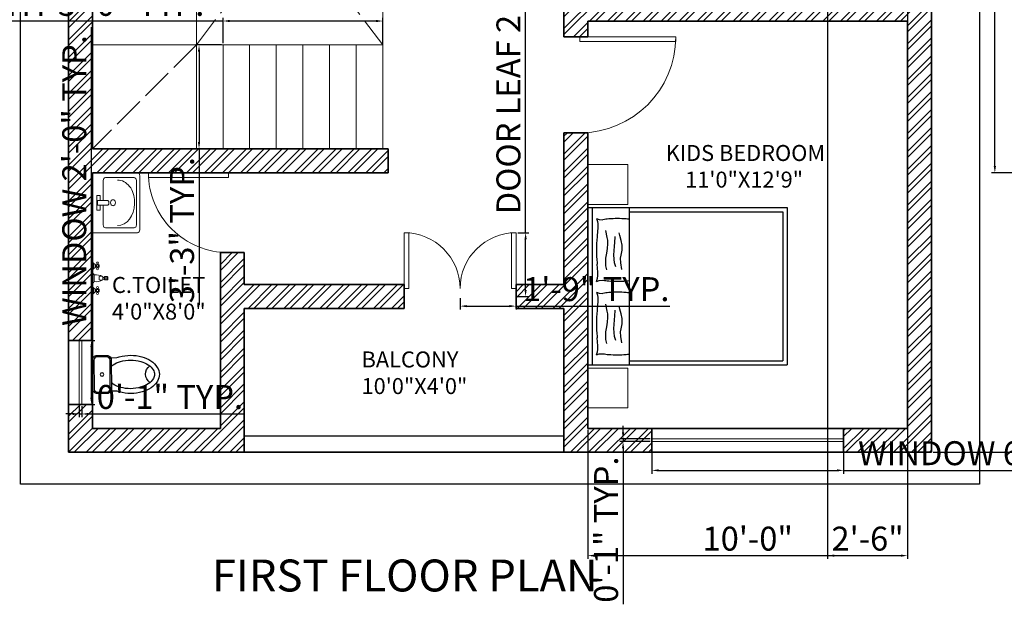
# Model space of a CAD drawing. Units: inches. Extents: x 638 to 1853, y 4393 to 5041.
# Tile 4 of 6: x 1072 to 1441, y 4399 to 4619. Entities that reach past the tile are written whole.
import ezdxf

# ---------------------------------------------------------------- set-up
doc = ezdxf.new("R2010")
doc.units = ezdxf.units.IN
doc.linetypes.add('ACAD_ISO02W100', pattern=[15, 12, -3])
for name, color, linetype, lineweight in [('A-ANNO-DIMS', 2, 'Continuous', 18), ('A-ANNO-TEXT', 7, 'Continuous', 25), ('A-AREA-IDEN', 7, 'Continuous', 18), ('A-DOOR', 4, 'Continuous', 18), ('A-FLOR-FIXT', 9, 'Continuous', 18), ('A-FLOR-STRS', 7, 'Continuous', 18), ('A-FLOR-STRS-HIDN', 7, 'ACAD_ISO02W100', 18), ('A-FURN', 26, 'Continuous', 13), ('A-GLAZ', 5, 'Continuous', 18), ('A-WALL', 7, 'Continuous', 35), ('A-WALL-PATT', 251, 'Continuous', 13), ('A-WALL-PRPT', 7, 'Continuous', 25), ('C-PROP', 7, 'Continuous', 25)]:
    doc.layers.add(name, color=color, linetype=linetype, lineweight=lineweight)
for name, color, linetype in [('SANTEH', 7, 'Continuous'), ('supurgelik', 31, 'Continuous'), ('TASLAR', 32, 'Continuous')]:
    doc.layers.add(name, color=color, linetype=linetype)
doc.styles.get("Standard").update_dxf_attribs({"font": 'arial.ttf'})
doc.dimstyles.new('ISO-25', dxfattribs={"dimtxt": 9, "dimasz": 2.5, "dimexe": 1.25, "dimexo": 0.625, "dimtad": 1, "dimdec": 1, "dimlunit": 3, "dimtxsty": 'Standard', "dimcen": 2.5, "dimadec": 0, "dimazin": 0, "dimtfac": 1, "dimtdec": 1, "dimtmove": 0, "dimatfit": 3, "dimfxl": 1, "dimarcsym": 0})

# ---------------------------------------------------------------- blocks, each defined once
blk = doc.blocks.new('*U2')
for p, q in [((0, 0), (0, -6)), ((-36, 0), (-36, -6))]:
    blk.add_line(p, q)
blk.add_lwpolyline([(0, 0), (0, 36), (-1.75, 36), (-1.75, 0)], close=True)
blk.add_arc((0, 0), 36, 90, 180)
blk = doc.blocks.new('*U3')
for p, q in [((-30, 0), (-30, -6)), ((0, 0), (0, -6))]:
    blk.add_line(p, q)
blk.add_lwpolyline([(0, 0), (0, 30), (-1.75, 30), (-1.75, 0)], close=True)
blk.add_arc((0, 0), 30, 90, 180)
blk = doc.blocks.new('hgjgh')
at = {"layer": 'supurgelik'}
for p, q in [((85993.81, -4751.89), (85843.81, -4751.89)), ((85853.26, -4756.05), (85856.29, -4757)), ((85853.26, -4756.05), (85854.18, -4758.49)), ((85854.18, -4758.49), (85854.49, -4762.19)), ((85856.29, -4757), (85858.52, -4757.5)), ((85858.52, -4757.5), (85862.12, -4757.37)), ((85862.12, -4757.37), (85869.57, -4756.72)), ((85904.4, -4757.37), (85896.95, -4756.72)), ((85908, -4757.5), (85904.4, -4757.37)), ((85910.23, -4757), (85908, -4757.5)), ((85913.26, -4756.05), (85910.23, -4757)), ((85912.34, -4758.49), (85912.03, -4762.19)), ((85913.26, -4756.05), (85912.34, -4758.49)), ((85923.48, -4756.05), (85926.51, -4757)), ((85923.48, -4756.05), (85924.4, -4758.49)), ((85924.4, -4758.49), (85924.71, -4762.19)), ((85926.51, -4757), (85928.74, -4757.5)), ((85928.74, -4757.5), (85932.34, -4757.37)), ((85932.34, -4757.37), (85939.79, -4756.72)), ((85974.62, -4757.37), (85967.17, -4756.72)), ((85978.22, -4757.5), (85974.62, -4757.37)), ((85980.45, -4757), (85978.22, -4757.5)), ((85983.48, -4756.05), (85980.45, -4757)), ((85982.56, -4758.49), (85982.25, -4762.19)), ((85983.48, -4756.05), (85982.56, -4758.49)), ((85864.23, -4765.86), (85867.95, -4764.99)), ((85867.95, -4764.99), (85871.91, -4764.87)), ((85871.91, -4764.87), (85875.39, -4765.12)), ((85875.39, -4765.12), (85878.49, -4765.74)), ((85878.49, -4765.74), (85881.96, -4766.23)), ((85881.96, -4766.23), (85884.81, -4766.61)), ((85884.81, -4766.61), (85888.65, -4766.85)), ((85888.65, -4766.85), (85892.62, -4766.85)), ((85892.62, -4766.85), (85895.1, -4766.36)), ((85895.1, -4766.36), (85901.8, -4764.87)), ((85934.44, -4765.86), (85938.16, -4764.99)), ((85938.16, -4764.99), (85942.13, -4764.87)), ((85942.13, -4764.87), (85945.6, -4765.12)), ((85945.6, -4765.12), (85948.7, -4765.74)), ((85948.7, -4765.74), (85952.18, -4766.23)), ((85952.18, -4766.23), (85955.03, -4766.61)), ((85955.03, -4766.61), (85958.87, -4766.85)), ((85958.87, -4766.85), (85962.84, -4766.85)), ((85962.84, -4766.85), (85965.32, -4766.36)), ((85965.32, -4766.36), (85972.02, -4764.87)), ((85871.29, -4773.05), (85867.33, -4774.04)), ((85870.92, -4779.28), (85875.39, -4779.03)), ((85874.27, -4772.55), (85871.29, -4773.05)), ((85878.86, -4772.3), (85874.27, -4772.55)), ((85875.39, -4779.03), (85878.24, -4779.65)), ((85881.96, -4772.55), (85878.86, -4772.3)), ((85887.04, -4773.05), (85881.96, -4772.55)), ((85890.14, -4773.3), (85887.04, -4773.05)), ((85896.09, -4773.67), (85890.14, -4773.3)), ((85892.37, -4779.65), (85896.96, -4778.41)), ((85896.96, -4778.41), (85899.69, -4777.54)), ((85941.51, -4773.05), (85937.54, -4774.04)), ((85941.14, -4779.28), (85945.6, -4779.03)), ((85944.49, -4772.55), (85941.51, -4773.05)), ((85949.08, -4772.3), (85944.49, -4772.55)), ((85945.6, -4779.03), (85948.46, -4779.65)), ((85952.18, -4772.55), (85949.08, -4772.3)), ((85957.26, -4773.05), (85952.18, -4772.55)), ((85960.36, -4773.3), (85957.26, -4773.05)), ((85966.31, -4773.67), (85960.36, -4773.3)), ((85962.59, -4779.65), (85967.18, -4778.41)), ((85967.18, -4778.41), (85969.91, -4777.54)), ((85993.81, -4787.2), (85843.81, -4787.2)), ((85847.81, -4787.2), (85847.81, -4933.89)), ((85864.72, -4780.15), (85870.92, -4779.28)), ((85878.24, -4779.65), (85882.95, -4780.4)), ((85882.95, -4780.4), (85887.91, -4780.4)), ((85887.91, -4780.4), (85892.37, -4779.65)), ((85934.94, -4780.15), (85941.14, -4779.28)), ((85948.46, -4779.65), (85953.17, -4780.4)), ((85953.17, -4780.4), (85958.13, -4780.4)), ((85958.13, -4780.4), (85962.59, -4779.65)), ((85989.81, -4787.2), (85989.81, -4933.89)), ((85989.81, -4933.89), (85847.81, -4933.89))]:
    blk.add_line(p, q, dxfattribs=at)
for centre, radius, start, end in [((85877.36, -4828.49), 72.19, 95.13619, 96.19323), ((85883.26, -4894.18), 138.14, 90, 95.13619), ((85883.26, -4894.18), 138.14, 84.86381, 90), ((85889.16, -4828.49), 72.19, 83.80677, 84.86381), ((85947.57, -4828.49), 72.19, 95.13619, 96.19323), ((85953.48, -4894.18), 138.14, 90, 95.13619), ((85953.48, -4894.18), 138.14, 84.86381, 90), ((85959.38, -4828.49), 72.19, 83.80677, 84.86381), ((85954.09, -4776.05), 100.71, 175.30047, 180), ((85905.8, -4772.08), 52.26, 169.08956, 175.30047), ((85860.72, -4772.08), 52.26, 4.69953, 10.91044), ((85812.43, -4776.05), 100.71, 0, 4.69953), ((86024.31, -4776.05), 100.71, 175.30047, 180), ((85976.02, -4772.08), 52.26, 169.08956, 175.30047), ((85930.94, -4772.08), 52.26, 4.69953, 10.91044), ((85882.65, -4776.05), 100.71, 0, 4.69953), ((85954.09, -4776.05), 100.71, 180, 184.69953), ((85812.43, -4776.05), 100.71, 355.30047, 0), ((86024.31, -4776.05), 100.71, 180, 184.69953), ((85882.65, -4776.05), 100.71, 355.30047, 0), ((85905.8, -4780.02), 52.26, 184.69953, 187.89725), ((85860.72, -4780.02), 52.26, 352.10275, 355.30047), ((85976.02, -4780.02), 52.26, 184.69953, 187.89725), ((85930.94, -4780.02), 52.26, 352.10275, 355.30047)]:
    blk.add_arc(centre, radius, start, end, dxfattribs=at)
at = {"layer": 'TASLAR'}
for p, q in [((85843.81, -4747.89), (85843.81, -4937.89)), ((85993.81, -4747.89), (85843.81, -4747.89)), ((85993.81, -4747.89), (85993.81, -4937.89)), ((85993.81, -4937.89), (85843.81, -4937.89))]:
    blk.add_line(p, q, dxfattribs=at)
blk = doc.blocks.new('K10-44')
at = {"layer": 'SANTEH'}
for points in [[(-182, 223, 0.020439), (-174, 198), (-174, 135, 0.262987), (-198, 92), (-198, -8, 0.414214), (-148, -58), (152, -58, 0.414214), (202, -8), (202, 92, 0.262987), (178, 135), (178, 198, 0.020439), (186, 223, 0.067459), (202, 342, 0.067459), (186, 461, 0.079812), (143, 554, 0.107118), (74, 621, 0.139889), (2, 642, 0.139889), (-70, 621, 0.107118), (-140, 554, 0.079812), (-182, 461, 0.067459), (-198, 342, 0.067459)], [(-148, 127), (152, 127, -0.414214), (187, 92), (187, -8, -0.414214), (152, -43), (-148, -43, -0.414214), (-183, -8), (-183, 92, -0.414214)]]:
    blk.add_lwpolyline(points, format="xyb", close=True, dxfattribs=at)
for points in [[(90, 142, 0.027307), (102, 158, 0.079812), (137, 236, 0.067459), (152, 342, 0.067459), (137, 448, 0.079812), (102, 526, 0.107118), (47, 579, 0.139889), (2, 592, 0.139889), (-44, 579, 0.107118), (-98, 526, 0.079812), (-134, 448, 0.067459), (-148, 342, 0.067459), (-134, 236, 0.079812), (-98, 158, 0.027307), (-86, 142, 0.139889)], [(-174, 135, -0.136371), (-148, 142), (152, 142, -0.136371), (178, 135)]]:
    blk.add_lwpolyline(points, format="xyb", dxfattribs=at)
blk.add_circle((2, 42), 18.3, dxfattribs=at)
blk.add_arc((2, 602), 105, 213.8994, 326.1006, dxfattribs=at)
blk = doc.blocks.new('Rac7')
at = {"color": 0}
for p, q in [((-39500.6, -24232.1), (-39500.6, -23829.6)), ((-39473.6, -23808.4), (-38988.3, -23808.4)), ((-39456.5, -23859.1), (-39456.5, -24114.9)), ((-39032.4, -23838), (-39429.6, -23838)), ((-39221.1, -23854.9), (-39240.8, -23854.9)), ((-39005.4, -24114.9), (-39005.4, -23859.1)), ((-39005.4, -23859.1), (-39005.4, -23859.1)), ((-38961.3, -23829.6), (-38961.3, -24232.1)), ((-39252.5, -24185.9), (-39252.5, -24093.6)), ((-39209.4, -24185.9), (-39209.4, -24093.6)), ((-39429.6, -24136.1), (-39252.5, -24136.1)), ((-39297, -24164), (-39252.5, -24164)), ((-39297, -24193.5), (-39297, -24164)), ((-39164.9, -24193.5), (-39297, -24193.5)), ((-39252.5, -24185.9), (-39209.4, -24185.9)), ((-39209.4, -24136.1), (-39032.4, -24136.1)), ((-39209.4, -24164), (-39164.9, -24164)), ((-39164.9, -24164), (-39164.9, -24193.5)), ((-38961.3, -24232.1), (-39500.6, -24232.1))]:
    blk.add_line(p, q, dxfattribs=at)
at = {"color": 0, "extrusion": (0, 0, -1)}
for centre, major_axis, start_param, end_param in [((-39473.6, -23829.6), (-27, 0), 0, 1.570796), ((-39429.6, -23859.1), (-27, 0), 0, 1.570796), ((-39240.8, -24007.4), (-194.1, 0), 0, 1.570796), ((-39221.1, -24007.4), (-194.1, 0), 1.570796, 3.141593), ((-39032.4, -23859.1), (-27, 0), 1.570796, 3.141593), ((-38988.3, -23829.6), (-27, 0), 1.570796, 3.141593), ((-39429.6, -24114.9), (-27, 0), -1.570796, 0), ((-39231, -24104), (-25.3, 0), 0.552816, 2.588777), ((-39032.4, -24114.9), (-27, 0), -3.141593, -1.570796)]:
    blk.add_ellipse(centre, major_axis=major_axis, ratio=0.785714, start_param=start_param, end_param=end_param, dxfattribs=at)
blk.add_ellipse((-39231, -24048), major_axis=(-27.9, 0), ratio=0.785714, dxfattribs=at)
blk = doc.blocks.new('Faucet - Bathroom front')
for p, q in [((-0.5, 4.25), (0.5, 4.25)), ((0.5, 3.75), (-0.5, 3.75)), ((-0.5, 3), (0.5, 3)), ((-0.25, 3), (-0.25, 3.5)), ((0.25, 3.5), (0.25, 3)), ((-5, 0), (-2.25, 0)), ((-4.5087, 0.25), (-2.7408, 0.25)), ((-4, 1.625), (-4.25, 1.625)), ((-4, 1.375), (-4.25, 1.375)), ((-3.1442, 0.75), (-4.0979, 0.75)), ((-3.25, 1.625), (-3, 1.625)), ((-3.25, 1.375), (-3, 1.375)), ((-1.5, 0), (1.5, 0)), ((-1, 0.5), (1, 0.5)), ((0.5, 2), (-0.5, 2)), ((2.25, 0), (5, 0)), ((2.7413, 0.25), (4.5092, 0.25)), ((3.25, 1.625), (3, 1.625)), ((3.25, 1.375), (3, 1.375)), ((4.1058, 0.75), (3.1521, 0.75)), ((4, 1.625), (4.25, 1.625)), ((4, 1.375), (4.25, 1.375))]:
    blk.add_line(p, q)
for points in [[(-0.5, 3.75), (-0.5, 4.25)], [(-0.25, 4.5), (0.25, 4.5)], [(0.25, 3.5), (-0.25, 3.5)], [(0.5, 4.25), (0.5, 3.75)]]:
    blk.add_lwpolyline(points)
for points in [[(-4, 1), (-4, 2), (-3.25, 2), (-3.25, 1)], [(3.25, 1), (3.25, 2), (4, 2), (4, 1)]]:
    blk.add_lwpolyline(points, close=True)
for centre in [(-4.5, 1.5), (-3.625, 1.5), (-2.75, 1.5), (2.75, 1.5), (3.625, 1.5), (4.5, 1.5)]:
    blk.add_circle(centre, 0.2795)
for centre, radius, start, end in [((3, 1), 4.0311, 150.2551, 187.125), ((0.6413, 2.5), 1.246, 156.3417, 203.6583), ((-0.2575, 4.2575), 0.2426, 88.22243, 181.7776), ((-0.2575, 3.7425), 0.2426, 178.2224, 271.7776), ((0.2575, 4.2575), 0.2426, 358.2224, 91.77757), ((0.2575, 3.7425), 0.2426, 268.2224, 1.777565), ((-3, 1), 4.0311, 352.875, 29.74488), ((-0.6413, 2.5), 1.246, 336.3417, 23.65835), ((-5.375, 1.375), 1.4252, 285.2551, 344.7449), ((-1.875, 1.375), 1.4252, 195.2551, 254.7449), ((-0.7962, -0.2038), 0.7327, 106.1502, 163.8498), ((0.7962, -0.2038), 0.7327, 16.1502, 73.84979), ((1.875, 1.375), 1.4252, 285.2551, 344.7449), ((5.375, 1.375), 1.4252, 195.2551, 254.7449)]:
    blk.add_arc(centre, radius, start, end)
blk = doc.blocks.new('BED-NIGHTSTAND-15')
blk.add_lwpolyline([(0, 14.98), (14.98, 14.98), (14.98, 0), (0, 0)], close=True)
blk = doc.blocks.new('WINDOW-GLAZING-24IN')
for p, q in [((0, 24), (0, 0)), ((1, 24), (1, 0))]:
    blk.add_line(p, q)
blk = doc.blocks.new('WINDOW-GLAZING-72IN')
for p, q in [((0, 72), (0, 0)), ((1, 72), (1, 0))]:
    blk.add_line(p, q)
blk = doc.blocks.new('DOOR-LEAF-21IN')
blk.add_line((21, 3), (21, 0))
blk.add_lwpolyline([(21, 3), (21, 24), (19.25, 24), (19.25, 3)], close=True)
blk.add_arc((21, 3), 21, 90, 180)
blk = doc.blocks.new('STAIR-WELL-OPENING')
for p, q in [((0, 93), (70, 0)), ((0, 0), (70, 93))]:
    blk.add_line(p, q)
blk.add_lwpolyline([(0, 93), (70, 93), (70, 0), (0, 0)], close=True)
blk = doc.blocks.new('STAIR-RUN-7-TREAD')
for p, q in [((0, 0), (0, 39)), ((10, 0), (10, 39)), ((20, 0), (20, 39)), ((30, 0), (30, 39)), ((40, 0), (40, 39)), ((50, 0), (50, 39)), ((60, 0), (60, 39))]:
    blk.add_line(p, q)
blk = doc.blocks.new('*D38')
at = {"layer": 'A-ANNO-DIMS', "color": 0, "lineweight": -2, "transparency": 16777216}
for p, q in [((1098.68, 4498.19), (1098.68, 4615.83)), ((1095.71, 4498.19), (1099.93, 4498.19)), ((1098.68, 4476.69), (1098.68, 4495.69)), ((1095.71, 4474.19), (1099.93, 4474.19))]:
    blk.add_line(p, q, dxfattribs=at)
at = {"layer": 'A-ANNO-DIMS', "color": 0, "transparency": 16777216}
for points in [[(1098.26, 4495.69), (1099.1, 4495.69), (1098.68, 4498.19)], [(1098.26, 4476.69), (1099.1, 4476.69), (1098.68, 4474.19)]]:
    blk.add_solid(points, dxfattribs=at)
at = {"layer": 'Defpoints', "color": 0, "transparency": 16777216}
for p in [(1095.08, 4498.19), (1098.68, 4498.19), (1095.08, 4474.19)]:
    blk.add_point(p, dxfattribs=at)
at = {"layer": 'A-ANNO-DIMS', "color": 0, "transparency": 16777216, "insert": (1093.4, 4558.26), "char_height": 9, "attachment_point": 5, "rotation": 90}
blk.add_mtext('WINDOW 2\'-0" TYP.', dxfattribs=at)
blk = doc.blocks.new('*D39')
at = {"layer": 'A-ANNO-DIMS', "color": 0, "lineweight": -2, "transparency": 16777216}
for p, q in [((1094.08, 4473.57), (1094.08, 4469.34)), ((1095.08, 4473.57), (1095.08, 4469.34)), ((1091.58, 4470.59), (1089.08, 4470.59)), ((1094.08, 4470.59), (1095.08, 4470.59)), ((1097.58, 4470.59), (1156.19, 4470.59))]:
    blk.add_line(p, q, dxfattribs=at)
at = {"layer": 'A-ANNO-DIMS', "color": 0, "transparency": 16777216}
for points in [[(1091.58, 4471.01), (1091.58, 4470.18), (1094.08, 4470.59)], [(1097.58, 4471.01), (1097.58, 4470.18), (1095.08, 4470.59)]]:
    blk.add_solid(points, dxfattribs=at)
at = {"layer": 'Defpoints', "color": 0, "transparency": 16777216}
for p in [(1094.08, 4474.19), (1095.08, 4474.19), (1095.08, 4470.59)]:
    blk.add_point(p, dxfattribs=at)
at = {"layer": 'A-ANNO-DIMS', "color": 0, "transparency": 16777216, "insert": (1128.14, 4475.81), "char_height": 9, "attachment_point": 5}
blk.add_mtext('0\'-1" TYP.', dxfattribs=at)
blk = doc.blocks.new('*D54')
at = {"layer": 'A-ANNO-DIMS', "color": 0, "lineweight": -2, "transparency": 16777216}
for p, q in [((1309.08, 4459.57), (1309.08, 4448.14)), ((1381.08, 4459.57), (1381.08, 4448.14)), ((1311.58, 4449.39), (1378.58, 4449.39)), ((1381.08, 4449.39), (1498.72, 4449.39))]:
    blk.add_line(p, q, dxfattribs=at)
at = {"layer": 'A-ANNO-DIMS', "color": 0, "transparency": 16777216}
for points in [[(1311.58, 4449.81), (1311.58, 4448.98), (1309.08, 4449.39)], [(1378.58, 4449.81), (1378.58, 4448.98), (1381.08, 4449.39)]]:
    blk.add_solid(points, dxfattribs=at)
at = {"layer": 'Defpoints', "color": 0, "transparency": 16777216}
for p in [(1309.08, 4460.19), (1381.08, 4460.19), (1381.08, 4449.39)]:
    blk.add_point(p, dxfattribs=at)
at = {"layer": 'A-ANNO-DIMS', "color": 0, "transparency": 16777216, "insert": (1441.15, 4454.68), "char_height": 9, "attachment_point": 5}
blk.add_mtext('WINDOW 6\'-0" TYP.', dxfattribs=at)
blk = doc.blocks.new('*D55')
at = {"layer": 'A-ANNO-DIMS', "color": 0, "lineweight": -2, "transparency": 16777216}
for p, q in [((1298.28, 4463.69), (1298.28, 4466.19)), ((1308.46, 4461.19), (1297.03, 4461.19)), ((1308.46, 4460.19), (1297.03, 4460.19)), ((1298.28, 4461.19), (1298.28, 4460.19)), ((1298.28, 4457.69), (1298.28, 4399.09))]:
    blk.add_line(p, q, dxfattribs=at)
at = {"layer": 'A-ANNO-DIMS', "color": 0, "transparency": 16777216}
for points in [[(1297.86, 4463.69), (1298.7, 4463.69), (1298.28, 4461.19)], [(1297.86, 4457.69), (1298.7, 4457.69), (1298.28, 4460.19)]]:
    blk.add_solid(points, dxfattribs=at)
at = {"layer": 'Defpoints', "color": 0, "transparency": 16777216}
for p in [(1298.28, 4460.19), (1309.08, 4461.19), (1309.08, 4460.19)]:
    blk.add_point(p, dxfattribs=at)
at = {"layer": 'A-ANNO-DIMS', "color": 0, "transparency": 16777216, "insert": (1293.06, 4427.14), "char_height": 9, "attachment_point": 5, "rotation": 90}
blk.add_mtext('0\'-1" TYP.', dxfattribs=at)
blk = doc.blocks.new('*D56')
at = {"layer": 'A-ANNO-DIMS', "color": 0, "lineweight": -2, "transparency": 16777216}
for p, q in [((1261.68, 4538.69), (1261.68, 4673.01)), ((1258.71, 4538.69), (1262.93, 4538.69)), ((1261.68, 4517.19), (1261.68, 4536.19)), ((1258.71, 4514.69), (1262.93, 4514.69))]:
    blk.add_line(p, q, dxfattribs=at)
at = {"layer": 'A-ANNO-DIMS', "color": 0, "transparency": 16777216}
for points in [[(1261.26, 4536.19), (1262.1, 4536.19), (1261.68, 4538.69)], [(1261.26, 4517.19), (1262.1, 4517.19), (1261.68, 4514.69)]]:
    blk.add_solid(points, dxfattribs=at)
at = {"layer": 'Defpoints', "color": 0, "transparency": 16777216}
for p in [(1258.08, 4538.69), (1261.68, 4538.69), (1258.08, 4514.69)]:
    blk.add_point(p, dxfattribs=at)
at = {"layer": 'A-ANNO-DIMS', "color": 0, "transparency": 16777216, "insert": (1256.4, 4607.1), "char_height": 9, "attachment_point": 5, "rotation": 90}
blk.add_mtext('DOOR LEAF 2\'-0" TYP.', dxfattribs=at)
blk = doc.blocks.new('*D57')
at = {"layer": 'A-ANNO-DIMS', "color": 0, "lineweight": -2, "transparency": 16777216}
for p, q in [((1237.08, 4514.07), (1237.08, 4509.84)), ((1258.08, 4514.07), (1258.08, 4509.84)), ((1239.58, 4511.09), (1255.58, 4511.09)), ((1258.08, 4511.09), (1315.84, 4511.09))]:
    blk.add_line(p, q, dxfattribs=at)
at = {"layer": 'A-ANNO-DIMS', "color": 0, "transparency": 16777216}
for points in [[(1239.58, 4511.51), (1239.58, 4510.68), (1237.08, 4511.09)], [(1255.58, 4511.51), (1255.58, 4510.68), (1258.08, 4511.09)]]:
    blk.add_solid(points, dxfattribs=at)
at = {"layer": 'Defpoints', "color": 0, "transparency": 16777216}
for p in [(1237.08, 4514.69), (1258.08, 4514.69), (1258.08, 4511.09)]:
    blk.add_point(p, dxfattribs=at)
at = {"layer": 'A-ANNO-DIMS', "color": 0, "transparency": 16777216, "insert": (1288.21, 4516.31), "char_height": 9, "attachment_point": 5}
blk.add_mtext('1\'-9" TYP.', dxfattribs=at)
blk = doc.blocks.new('*D58')
at = {"layer": 'A-ANNO-DIMS', "color": 0, "lineweight": -2, "transparency": 16777216}
for p, q in [((1148.08, 4618.19), (1000.8, 4618.19)), ((1148.08, 4609.82), (1148.08, 4619.44)), ((1205.58, 4618.19), (1150.58, 4618.19)), ((1208.08, 4609.82), (1208.08, 4619.44))]:
    blk.add_line(p, q, dxfattribs=at)
at = {"layer": 'A-ANNO-DIMS', "color": 0, "transparency": 16777216}
for points in [[(1150.58, 4618.61), (1150.58, 4617.78), (1148.08, 4618.19)], [(1205.58, 4618.61), (1205.58, 4617.78), (1208.08, 4618.19)]]:
    blk.add_solid(points, dxfattribs=at)
at = {"layer": 'Defpoints', "color": 0, "transparency": 16777216}
for p in [(1148.08, 4618.19), (1148.08, 4609.19), (1208.08, 4609.19)]:
    blk.add_point(p, dxfattribs=at)
at = {"layer": 'A-ANNO-DIMS', "color": 0, "transparency": 16777216, "insert": (1073.19, 4623.47), "char_height": 9, "attachment_point": 5}
blk.add_mtext('STAIR FLIGHT 5\'-0" TYP.', dxfattribs=at)
blk = doc.blocks.new('*D59')
at = {"layer": 'A-ANNO-DIMS', "color": 0, "lineweight": -2, "transparency": 16777216}
for p, q in [((1147.46, 4609.19), (1137.83, 4609.19)), ((1139.08, 4606.69), (1139.08, 4572.69)), ((1147.46, 4570.19), (1137.83, 4570.19)), ((1139.08, 4570.19), (1139.08, 4511.59))]:
    blk.add_line(p, q, dxfattribs=at)
at = {"layer": 'A-ANNO-DIMS', "color": 0, "transparency": 16777216}
for points in [[(1138.66, 4606.69), (1139.5, 4606.69), (1139.08, 4609.19)], [(1138.66, 4572.69), (1139.5, 4572.69), (1139.08, 4570.19)]]:
    blk.add_solid(points, dxfattribs=at)
at = {"layer": 'Defpoints', "color": 0, "transparency": 16777216}
for p in [(1148.08, 4609.19), (1139.08, 4570.19), (1148.08, 4570.19)]:
    blk.add_point(p, dxfattribs=at)
at = {"layer": 'A-ANNO-DIMS', "color": 0, "transparency": 16777216, "insert": (1133.86, 4539.64), "char_height": 9, "attachment_point": 5, "rotation": 90}
blk.add_mtext('3\'-3" TYP.', dxfattribs=at)
blk = doc.blocks.new('*D89')
at = {"layer": 'A-ANNO-DIMS', "color": 0, "lineweight": -2, "transparency": 16777216}
for p, q in [((1414.71, 4906.19), (1460.16, 4906.19)), ((1458.91, 4458.69), (1458.91, 4903.69)), ((1414.71, 4456.19), (1460.16, 4456.19))]:
    blk.add_line(p, q, dxfattribs=at)
at = {"layer": 'A-ANNO-DIMS', "color": 0, "transparency": 16777216}
for points in [[(1458.49, 4903.69), (1459.32, 4903.69), (1458.91, 4906.19)], [(1458.49, 4458.69), (1459.32, 4458.69), (1458.91, 4456.19)]]:
    blk.add_solid(points, dxfattribs=at)
at = {"layer": 'Defpoints', "color": 0, "transparency": 16777216}
for p in [(1414.08, 4906.19), (1458.91, 4906.19), (1414.08, 4456.19)]:
    blk.add_point(p, dxfattribs=at)
at = {"layer": 'A-ANNO-DIMS', "color": 0, "transparency": 16777216, "insert": (1453.68, 4681.19), "char_height": 9, "attachment_point": 5, "rotation": 90}
blk.add_mtext('37\'-6"', dxfattribs=at)
blk = doc.blocks.new('*D90')
at = {"layer": 'A-ANNO-DIMS', "color": 0, "lineweight": -2, "transparency": 16777216}
for p, q in [((1285.08, 4464.57), (1285.08, 4416.12)), ((1405.08, 4464.57), (1405.08, 4416.12)), ((1287.58, 4417.37), (1402.58, 4417.37))]:
    blk.add_line(p, q, dxfattribs=at)
at = {"layer": 'A-ANNO-DIMS', "color": 0, "transparency": 16777216}
for points in [[(1287.58, 4417.79), (1287.58, 4416.95), (1285.08, 4417.37)], [(1402.58, 4417.79), (1402.58, 4416.95), (1405.08, 4417.37)]]:
    blk.add_solid(points, dxfattribs=at)
at = {"layer": 'Defpoints', "color": 0, "transparency": 16777216}
for p in [(1285.08, 4465.19), (1405.08, 4465.19), (1405.08, 4417.37)]:
    blk.add_point(p, dxfattribs=at)
at = {"layer": 'A-ANNO-DIMS', "color": 0, "transparency": 16777216, "insert": (1345.08, 4422.59), "char_height": 9, "attachment_point": 5}
blk.add_mtext('10\'-0"', dxfattribs=at)
blk = doc.blocks.new('*D92')
at = {"layer": 'A-ANNO-DIMS', "color": 0, "lineweight": -2, "transparency": 16777216}
for p, q in [((1375.08, 4755.57), (1375.08, 4416.12)), ((1405.08, 4755.57), (1405.08, 4416.12)), ((1377.58, 4417.37), (1402.58, 4417.37))]:
    blk.add_line(p, q, dxfattribs=at)
at = {"layer": 'A-ANNO-DIMS', "color": 0, "transparency": 16777216}
for points in [[(1377.58, 4417.79), (1377.58, 4416.95), (1375.08, 4417.37)], [(1402.58, 4417.79), (1402.58, 4416.95), (1405.08, 4417.37)]]:
    blk.add_solid(points, dxfattribs=at)
at = {"layer": 'Defpoints', "color": 0, "transparency": 16777216}
for p in [(1375.08, 4756.19), (1405.08, 4756.19), (1405.08, 4417.37)]:
    blk.add_point(p, dxfattribs=at)
at = {"layer": 'A-ANNO-DIMS', "color": 0, "transparency": 16777216, "insert": (1390.08, 4422.59), "char_height": 9, "attachment_point": 5}
blk.add_mtext('2\'-6"', dxfattribs=at)
blk = doc.blocks.new('*D97')
at = {"layer": 'A-ANNO-DIMS', "color": 0, "lineweight": -2, "transparency": 16777216}
for p, q in [((1482.06, 4906.19), (1436.61, 4906.19)), ((1437.86, 4563.69), (1437.86, 4903.69)), ((1482.06, 4561.19), (1436.61, 4561.19))]:
    blk.add_line(p, q, dxfattribs=at)
at = {"layer": 'A-ANNO-DIMS', "color": 0, "transparency": 16777216}
for points in [[(1437.44, 4903.69), (1438.27, 4903.69), (1437.86, 4906.19)], [(1437.44, 4563.69), (1438.27, 4563.69), (1437.86, 4561.19)]]:
    blk.add_solid(points, dxfattribs=at)
at = {"layer": 'Defpoints', "color": 0, "transparency": 16777216}
for p in [(1437.86, 4906.19), (1482.68, 4906.19), (1482.68, 4561.19)]:
    blk.add_point(p, dxfattribs=at)
at = {"layer": 'A-ANNO-DIMS', "color": 0, "transparency": 16777216, "insert": (1432.64, 4733.69), "char_height": 9, "attachment_point": 5, "rotation": 90}
blk.add_mtext('28\'-9"', dxfattribs=at)

msp = doc.modelspace()

# ---------------------------------------------------------------- hatches: boundary and pattern name
at = {"layer": 'A-WALL-PATT', "transparency": 33554687}
h = msp.add_hatch(dxfattribs=at)
h.set_pattern_fill('ANSI32', color=256, scale=0.5)
h.set_pattern_definition([(45, (-45.7406, 0), (-3.367596, 3.367596), []), (45, (-43.4956, 0), (-3.367596, 3.367596), [])])
h.paths.add_polyline_path([(1414.08, 4693.19), (1405.08, 4693.19), (1405.08, 4627.19), (1285.08, 4627.19), (1285.08, 4633.19), (1282.08, 4633.19), (1276.08, 4633.19), (1276.08, 4612.19), (1282.08, 4612.19), (1285.08, 4612.19), (1285.08, 4618.19), (1405.08, 4618.19), (1405.08, 4465.19), (1381.08, 4465.19), (1381.08, 4456.19), (1414.08, 4456.19)])
h.paths.add_polyline_path([(1216.08, 4519.19), (1156.08, 4519.19), (1156.08, 4531.19), (1150.08, 4531.19), (1147.08, 4531.19), (1147.08, 4465.19), (1099.08, 4465.19), (1099.08, 4474.19), (1090.08, 4474.19), (1090.08, 4456.19), (1156.08, 4456.19), (1156.08, 4510.19), (1216.08, 4510.19)])
h.paths.add_polyline_path([(1285.08, 4576.19), (1276.08, 4576.19), (1276.08, 4519.19), (1258.08, 4519.19), (1258.08, 4517.69), (1258.08, 4514.69), (1258.08, 4510.19), (1276.08, 4510.19), (1276.08, 4456.19), (1309.08, 4456.19), (1309.08, 4465.19), (1285.08, 4465.19)])
h.paths.add_polyline_path([(1414.08, 4780.19), (1405.08, 4780.19), (1405.08, 4762.19), (1405.08, 4756.19), (1405.08, 4747.19), (1414.08, 4747.19)], flags=17)
h.paths.add_polyline_path([(1414.08, 4906.19), (1339.08, 4906.19), (1339.08, 4897.19), (1369.08, 4897.19), (1369.08, 4855.19), (1375.08, 4855.19), (1375.08, 4897.19), (1405.08, 4897.19), (1405.08, 4825.19), (1276.08, 4825.19), (1276.08, 4765.19), (1270.08, 4765.19), (1270.08, 4756.19), (1276.08, 4756.19), (1276.08, 4669.19), (1285.08, 4669.19), (1285.08, 4756.19), (1375.08, 4756.19), (1375.08, 4765.19), (1285.08, 4765.19), (1285.08, 4819.19), (1405.08, 4819.19), (1405.08, 4804.19), (1414.08, 4804.19)])
h.paths.add_polyline_path([(1315.08, 4906.19), (1222.08, 4906.19), (1222.08, 4897.19), (1233.28, 4897.19), (1276.08, 4897.19), (1276.08, 4855.19), (1282.08, 4855.19), (1285.08, 4855.19), (1285.08, 4897.19), (1307.64, 4897.19), (1315.08, 4897.19)])
h.paths.add_polyline_path([(1099.08, 4897.19), (1168.08, 4897.19), (1168.08, 4906.19), (1090.08, 4906.19), (1090.08, 4498.19), (1099.08, 4498.19), (1099.08, 4561.19), (1115.92, 4561.19), (1210.08, 4561.19), (1210.08, 4570.19), (1099.08, 4570.19), (1099.08, 4756.19), (1234.08, 4756.19), (1234.08, 4762.19), (1234.08, 4765.19), (1099.08, 4765.19)])
h.paths.add_polyline_path([(1312.08, 4654.44), (1389.59, 4654.44), (1389.59, 4676.83), (1312.08, 4676.83)], flags=25)
h.paths.add_polyline_path([(1302.5, 4782.68), (1343.68, 4782.68), (1343.68, 4805.07), (1302.5, 4805.07)], flags=25)
h.paths.add_polyline_path([(1298.34, 4860.64), (1339, 4860.64), (1339, 4883.02), (1298.34, 4883.02)], flags=25)

# ---------------------------------------------------------------- linework, layer by layer
at = {"layer": 'A-FLOR-STRS'}
for p, q in [((1138.08, 4570.19), (1138.08, 4719.19)), ((1208.08, 4609.19), (1099.08, 4609.19))]:
    msp.add_line(p, q, dxfattribs=at)
at = {"layer": 'A-FLOR-STRS-HIDN'}
msp.add_line((1138.08, 4609.19), (1099.08, 4570.19), dxfattribs=at)
at = {"layer": 'A-WALL'}
for p, q in [((1090.08, 4456.19), (1090.08, 4906.19)), ((1414.08, 4906.19), (1414.08, 4456.19)), ((1099.08, 4570.19), (1099.08, 4756.19)), ((1276.08, 4612.19), (1276.08, 4633.19)), ((1405.08, 4618.19), (1285.08, 4618.19)), ((1285.08, 4612.19), (1285.08, 4618.19)), ((1405.08, 4618.19), (1405.08, 4465.19)), ((1285.08, 4612.19), (1276.08, 4612.19)), ((1285.08, 4576.19), (1276.08, 4576.19)), ((1276.08, 4519.19), (1276.08, 4576.19)), ((1285.08, 4465.19), (1285.08, 4576.19)), ((1210.08, 4570.19), (1099.08, 4570.19)), ((1210.08, 4561.19), (1210.08, 4570.19)), ((1210.08, 4561.19), (1099.08, 4561.19)), ((1099.08, 4465.19), (1099.08, 4561.19)), ((1156.08, 4531.19), (1147.08, 4531.19)), ((1147.08, 4465.19), (1147.08, 4531.19)), ((1156.08, 4519.19), (1156.08, 4531.19)), ((1216.08, 4519.19), (1156.08, 4519.19)), ((1216.08, 4510.19), (1216.08, 4519.19)), ((1276.08, 4519.19), (1258.08, 4519.19)), ((1258.08, 4510.19), (1258.08, 4519.19)), ((1216.08, 4510.19), (1156.08, 4510.19)), ((1156.08, 4456.19), (1156.08, 4510.19)), ((1276.08, 4510.19), (1258.08, 4510.19)), ((1276.08, 4456.19), (1276.08, 4510.19)), ((1099.08, 4498.19), (1090.08, 4498.19)), ((1099.08, 4474.19), (1090.08, 4474.19)), ((1147.08, 4465.19), (1099.08, 4465.19)), ((1405.08, 4465.19), (1285.08, 4465.19)), ((1309.08, 4465.19), (1309.08, 4456.19)), ((1381.08, 4465.19), (1381.08, 4456.19)), ((1414.08, 4456.19), (1090.08, 4456.19))]:
    msp.add_line(p, q, dxfattribs=at)
at = {"layer": 'A-WALL-PRPT'}
msp.add_line((1276.08, 4462.19), (1156.08, 4462.19), dxfattribs=at)
at = {"layer": 'C-PROP'}
msp.add_lwpolyline([(1072.08, 4924.19), (1432.08, 4924.19), (1432.08, 4444.19), (1072.08, 4444.19)], close=True, dxfattribs=at)

# ---------------------------------------------------------------- block references
at = {"layer": 'A-DOOR', "xscale": -1, "rotation": 270}
msp.add_blockref('*U2', (1282.08, 4612.19), dxfattribs=at)
at = {"layer": 'A-DOOR', "rotation": 89.99999999999999}
msp.add_blockref('*U3', (1150.08, 4561.19), dxfattribs=at)
at = {"layer": 'A-DOOR', "extrusion": (0, 0, -1), "zscale": -1}
msp.add_blockref('DOOR-LEAF-21IN', (-1237.08, 4514.69), dxfattribs=at)
at = {"layer": 'A-DOOR'}
msp.add_blockref('DOOR-LEAF-21IN', (1237.08, 4514.69), dxfattribs=at)
at = {"layer": 'A-FLOR-FIXT'}
for name, p, xscale, yscale, zscale, rotation in [('Rac7', (2112.7, 6190.93), -0.0418294453001151, 0.0418294453001151, 0.0418294453001151, 270), ('Faucet - Bathroom front', (1099.08, 4521.57), 1.274234813154425, 1.274234813154425, 1.274234813154425, 270), ('K10-44', (1101.16, 4485.32), -0.0358529150226637, 0.0358529150226637, 0.0358529150226637, 270.3279556026283)]:
    msp.add_blockref(name, p, dxfattribs=dict(at, xscale=xscale, yscale=yscale, zscale=zscale, rotation=rotation))
at = {"layer": 'A-FLOR-STRS', "rotation": 180}
msp.add_blockref('STAIR-RUN-7-TREAD', (1208.08, 4609.19), dxfattribs=at)
at = {"layer": 'A-FLOR-STRS-HIDN'}
msp.add_blockref('STAIR-WELL-OPENING', (1138.08, 4609.19), dxfattribs=at)
at = {"layer": 'A-FURN', "rotation": 90.00000000364122}
msp.add_blockref('BED-NIGHTSTAND-15', (1300.07, 4549.28), dxfattribs=at)
at = {"layer": 'A-FURN', "xscale": 0.393701, "yscale": 0.393701, "zscale": 0.393701, "rotation": 90}
msp.add_blockref('hgjgh', (-584.17, -29307.76), dxfattribs=at)
at = {"layer": 'A-FURN'}
msp.add_blockref('BED-NIGHTSTAND-15', (1285.08, 4472.87), dxfattribs=at)
at = {"layer": 'A-GLAZ'}
msp.add_blockref('WINDOW-GLAZING-24IN', (1094.08, 4474.19), dxfattribs=at)
at = {"layer": 'A-GLAZ', "rotation": 270.0000000000014}
msp.add_blockref('WINDOW-GLAZING-72IN', (1309.08, 4461.19), dxfattribs=at)

# ---------------------------------------------------------------- texts
at = {"layer": 'A-ANNO-TEXT', "insert": (1143.93, 4415.91), "char_height": 12, "attachment_point": 1}
msp.add_mtext_dynamic_manual_height_columns('FIRST FLOOR PLAN', width=193.1285, gutter_width=12.5, heights=[0], dxfattribs=at)
at = {"layer": 'A-AREA-IDEN', "char_height": 6, "attachment_point": 1}
for s, width, insert in [('KIDS BEDROOM\\P    11\'0"X12\'9"', 125.7999, (1314.26, 4571.62)), ('\\pxt3;C.TOILET\\P4\'0"X8\'0"', 77.4832, (1106.39, 4522.04)), ('\\pxt3;BALCONY\\P10\'0"X4\'0"', 77.4832, (1200.09, 4494.07))]:
    msp.add_mtext_dynamic_manual_height_columns(s, width=width, gutter_width=12.5, heights=[0], dxfattribs=dict(at, insert=insert))

# ---------------------------------------------------------------- dimensions: what is measured, and where the dimension line sits
at = {"layer": 'A-ANNO-DIMS'}
for base, p1, p2, picture, middle in [((1458.91, 4906.19), (1414.08, 4456.19), (1414.08, 4906.19), '*D89', (1453.68, 4681.19)), ((1437.86, 4906.19), (1482.68, 4561.19), (1482.68, 4906.19), '*D97', (1432.64, 4733.69))]:
    dim = msp.add_linear_dim(base=base, p1=p1, p2=p2, angle=90, dimstyle='ISO-25', override={"dimdec": 1, "dimlfac": 1, "dimrnd": 0, "dimzin": 1, "dimdsep": 46, "dimlunit": 4, "dimfrac": 2}, dxfattribs=at)
    dim.commit()
    dim.dimension.update_dxf_attribs({"geometry": picture, "text_midpoint": middle})
for p1, p2, picture, middle in [((1375.08, 4756.19), (1405.08, 4756.19), '*D92', (1390.08, 4422.59)), ((1285.08, 4465.19), (1405.08, 4465.19), '*D90', (1345.08, 4422.59))]:
    dim = msp.add_linear_dim(base=(1405.08, 4417.37), p1=p1, p2=p2, dimstyle='ISO-25', override={"dimdec": 1, "dimlfac": 1, "dimrnd": 0, "dimzin": 1, "dimdsep": 46, "dimlunit": 4, "dimfrac": 2}, dxfattribs=at)
    dim.commit()
    dim.dimension.update_dxf_attribs({"geometry": picture, "text_midpoint": middle})
for base, p1, p2, angle, text, picture, middle in [((1261.68, 4538.69), (1258.08, 4514.69), (1258.08, 4538.69), 90, 'DOOR LEAF <> TYP.', '*D56', (1256.4, 4607.1)), ((1148.08, 4618.19), (1208.08, 4609.19), (1148.08, 4609.19), 180, 'STAIR FLIGHT <> TYP.', '*D58', (1073.19, 4623.47)), ((1098.68, 4498.19), (1095.08, 4474.19), (1095.08, 4498.19), 90, 'WINDOW <> TYP.', '*D38', (1093.4, 4558.26)), ((1139.08, 4570.19), (1148.08, 4609.19), (1148.08, 4570.19), 270, '<> TYP.', '*D59', (1133.86, 4539.64)), ((1381.08, 4449.39), (1309.08, 4460.19), (1381.08, 4460.19), 0, 'WINDOW <> TYP.', '*D54', (1441.15, 4454.68)), ((1298.28, 4460.19), (1309.08, 4461.19), (1309.08, 4460.19), 270, '<> TYP.', '*D55', (1293.06, 4427.14))]:
    dim = msp.add_linear_dim(base=base, p1=p1, p2=p2, angle=angle, text=text, dimstyle='ISO-25', override={"dimdec": 1, "dimlfac": 1, "dimrnd": 0, "dimzin": 1, "dimdsep": 46, "dimlunit": 4, "dimfrac": 2}, dxfattribs=at)
    dim.commit()
    dim.dimension.update_dxf_attribs({"geometry": picture, "text_midpoint": middle})
for base, p1, p2, picture, middle in [((1258.08, 4511.09), (1237.08, 4514.69), (1258.08, 4514.69), '*D57', (1288.21, 4516.31)), ((1095.08, 4470.59), (1094.08, 4474.19), (1095.08, 4474.19), '*D39', (1128.14, 4475.81))]:
    dim = msp.add_linear_dim(base=base, p1=p1, p2=p2, text='<> TYP.', dimstyle='ISO-25', override={"dimdec": 1, "dimlfac": 1, "dimrnd": 0, "dimzin": 1, "dimdsep": 46, "dimlunit": 4, "dimfrac": 2}, dxfattribs=at)
    dim.commit()
    dim.dimension.update_dxf_attribs({"geometry": picture, "text_midpoint": middle})

doc.saveas('drawing.dxf')
